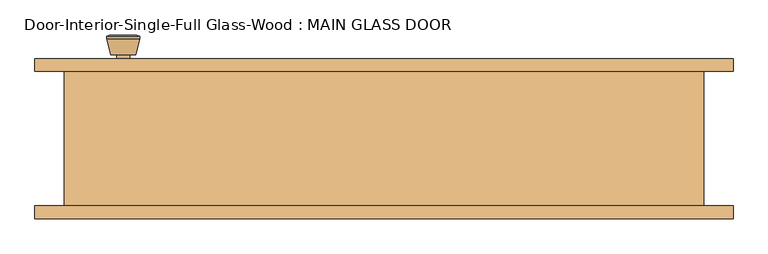
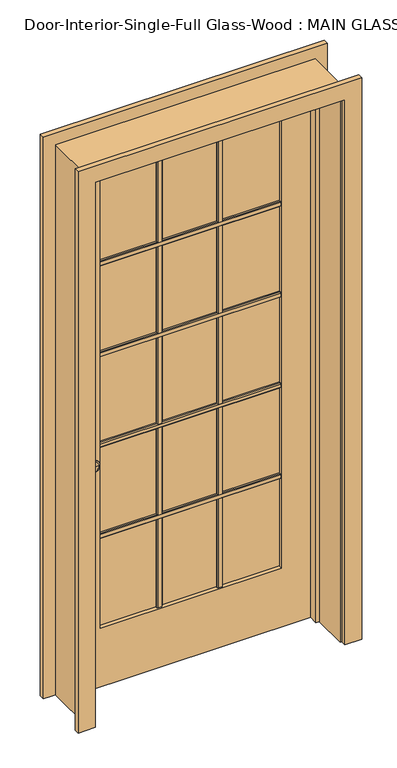
"""IFC4 building model written with IfcOpenShell, lengths in millimetres: door geometry, Door-Interior-Single-Full Glass-Wood : MAIN GLASS DOOR."""

from ifc_helpers import new_model, si_unit, point, frame, frame_2d, origin, place, context, project, spatial, polyline, circle_curve, trimmed, segment, composite_curve, outline, extrude, faceted_brep, source, transform, mapped, element, save
from ifc_brep_helpers import plane_surface, cylinder_surface, revolved_surface, advanced_brep


def door_interior_single_full_glass_wood_main_glass_door_aaee7461(model_context):
    return source(origin(), model_context, "Body", "SolidModel", [
        extrude(outline(polyline([(84.455, 1667.51), (90.805, 1667.51), (93.98, 1664.335), (93.98, 1651.635), (90.805, 1648.46), (84.455, 1648.46), (84.455, 1667.51)])), frame((-336.55, 0.0, 0.0), z_axis=(1.0, 0.0, 0.0), x_axis=(0.0, 1.0, 0.0)), (0.0, 0.0, 1.0), 673.1),
        extrude(outline(polyline([(84.455, 1310.9575), (90.805, 1310.9575), (93.98, 1307.7825), (93.98, 1295.0825), (90.805, 1291.9075), (84.455, 1291.9075), (84.455, 1310.9575)])), frame((-336.55, 0.0, 0.0), z_axis=(1.0, 0.0, 0.0), x_axis=(0.0, 1.0, 0.0)), (0.0, 0.0, 1.0), 673.1),
        extrude(outline(polyline([(84.455, 954.405), (90.805, 954.405), (93.98, 951.23), (93.98, 938.53), (90.805, 935.355), (84.455, 935.355), (84.455, 954.405)])), frame((-336.55, 0.0, 0.0), z_axis=(1.0, 0.0, 0.0), x_axis=(0.0, 1.0, 0.0)), (0.0, 0.0, 1.0), 673.1),
        extrude(outline(polyline([(84.455, 597.8525), (90.805, 597.8525), (93.98, 594.6775), (93.98, 581.9775), (90.805, 578.8025), (84.455, 578.8025), (84.455, 597.8525)])), frame((-336.55, 0.0, 0.0), z_axis=(1.0, 0.0, 0.0), x_axis=(0.0, 1.0, 0.0)), (0.0, 0.0, 1.0), 673.1),
        extrude(outline(polyline([(102.6583333, 84.455), (102.6583333, 90.805), (105.8333333, 93.98), (118.5333333, 93.98), (121.7083333, 90.805), (121.7083333, 84.455), (102.6583333, 84.455)])), frame((0.0, 0.0, 231.775), z_axis=(0.0, 0.0, 1.0), x_axis=(1.0, 0.0, 0.0)), (0.0, 0.0, 1.0), 1782.7625),
        extrude(outline(polyline([(-121.7083333, 84.455), (-121.7083333, 90.805), (-118.5333333, 93.98), (-105.8333333, 93.98), (-102.6583333, 90.805), (-102.6583333, 84.455), (-121.7083333, 84.455)])), frame((0.0, 0.0, 231.775), z_axis=(0.0, 0.0, 1.0), x_axis=(1.0, 0.0, 0.0)), (0.0, 0.0, 1.0), 1782.7625),
        extrude(outline(polyline([(77.47, 1667.51), (77.47, 1648.46), (71.12, 1648.46), (67.945, 1651.635), (67.945, 1664.335), (71.12, 1667.51), (77.47, 1667.51)])), frame((-336.55, 0.0, 0.0), z_axis=(1.0, 0.0, 0.0), x_axis=(0.0, 1.0, 0.0)), (0.0, 0.0, 1.0), 673.1),
        extrude(outline(polyline([(77.47, 1310.9575), (77.47, 1291.9075), (71.12, 1291.9075), (67.945, 1295.0825), (67.945, 1307.7825), (71.12, 1310.9575), (77.47, 1310.9575)])), frame((-336.55, 0.0, 0.0), z_axis=(1.0, 0.0, 0.0), x_axis=(0.0, 1.0, 0.0)), (0.0, 0.0, 1.0), 673.1),
        extrude(outline(polyline([(77.47, 954.405), (77.47, 935.355), (71.12, 935.355), (67.945, 938.53), (67.945, 951.23), (71.12, 954.405), (77.47, 954.405)])), frame((-336.55, 0.0, 0.0), z_axis=(1.0, 0.0, 0.0), x_axis=(0.0, 1.0, 0.0)), (0.0, 0.0, 1.0), 673.1),
        extrude(outline(polyline([(77.47, 597.8525), (77.47, 578.8025), (71.12, 578.8025), (67.945, 581.9775), (67.945, 594.6775), (71.12, 597.8525), (77.47, 597.8525)])), frame((-336.55, 0.0, 0.0), z_axis=(1.0, 0.0, 0.0), x_axis=(0.0, 1.0, 0.0)), (0.0, 0.0, 1.0), 673.1),
        extrude(outline(polyline([(102.6583333, 77.47), (121.7083333, 77.47), (121.7083333, 71.12), (118.5333333, 67.945), (105.8333333, 67.945), (102.6583333, 71.12), (102.6583333, 77.47)])), frame((0.0, 0.0, 231.775), z_axis=(0.0, 0.0, 1.0), x_axis=(1.0, 0.0, 0.0)), (0.0, 0.0, 1.0), 1782.7625),
        extrude(outline(polyline([(-121.7083333, 77.47), (-102.6583333, 77.47), (-102.6583333, 71.12), (-105.8333333, 67.945), (-118.5333333, 67.945), (-121.7083333, 71.12), (-121.7083333, 77.47)])), frame((0.0, 0.0, 231.775), z_axis=(0.0, 0.0, 1.0), x_axis=(1.0, 0.0, 0.0)), (0.0, 0.0, 1.0), 1782.7625),
        advanced_brep(
        [(-393.7, 57.5, 914.4), (-383.7, 57.5, 914.4), (-403.7, 57.5, 914.4), (-373.2241324, 8.5, 914.4), (-393.7, 8.5, 914.4), (-414.1758676, 8.5, 914.4), (-368.7, 10.3278681, 914.4), (-418.7, 10.3278681, 914.4), (-368.7, 13.7915463, 914.4), (-418.7, 13.7915463, 914.4), (-375.063764, 38.5, 914.4), (-412.336236, 38.5, 914.4), (-383.7, 38.5, 914.4), (-403.7, 38.5, 914.4)],
        [
            (0, 1),
            (1, 2, circle_curve(frame((-393.7, 57.5, 914.4), z_axis=(0.0, 1.0, 0.0), x_axis=(-1.0, 0.0, 0.0)), 10.0)),
            (2, 0),
            (2, 1, circle_curve(frame((-393.7, 57.5, 914.4), z_axis=(0.0, 1.0, 0.0), x_axis=(-1.0, 0.0, 0.0)), 10.0)),
            (3, 4),
            (4, 5),
            (5, 3, circle_curve(frame((-393.7, 8.5, 914.4), z_axis=(0.0, -1.0, 0.0), x_axis=(-1.0, 0.0, 0.0)), 20.4758676)),
            (3, 5, circle_curve(frame((-393.7, 8.5, 914.4), z_axis=(0.0, -1.0, 0.0), x_axis=(-1.0, 0.0, 0.0)), 20.4758676)),
            (6, 3),
            (5, 7),
            (7, 6, circle_curve(frame((-393.7, 10.3278681, 914.4), z_axis=(0.0, -1.0, 0.0), x_axis=(-1.0, 0.0, 0.0)), 25.0)),
            (6, 7, circle_curve(frame((-393.7, 10.3278681, 914.4), z_axis=(0.0, -1.0, 0.0), x_axis=(-1.0, 0.0, 0.0)), 25.0)),
            (8, 6),
            (7, 9),
            (9, 8, circle_curve(frame((-393.7, 13.7915463, 914.4), z_axis=(0.0, -1.0, 0.0), x_axis=(-1.0, 0.0, 0.0)), 25.0)),
            (8, 9, circle_curve(frame((-393.7, 13.7915463, 914.4), z_axis=(0.0, -1.0, 0.0), x_axis=(-1.0, 0.0, 0.0)), 25.0)),
            (10, 8),
            (9, 11),
            (11, 10, circle_curve(frame((-393.7, 38.5, 914.4), z_axis=(0.0, -1.0, 0.0), x_axis=(-1.0, 0.0, 0.0)), 18.636236)),
            (10, 11, circle_curve(frame((-393.7, 38.5, 914.4), z_axis=(0.0, -1.0, 0.0), x_axis=(-1.0, 0.0, 0.0)), 18.636236)),
            (12, 10),
            (11, 13),
            (13, 12, circle_curve(frame((-393.7, 38.5, 914.4), z_axis=(0.0, -1.0, 0.0), x_axis=(-1.0, 0.0, 0.0)), 10.0)),
            (12, 13, circle_curve(frame((-393.7, 38.5, 914.4), z_axis=(0.0, -1.0, 0.0), x_axis=(-1.0, 0.0, 0.0)), 10.0)),
            (1, 12),
            (13, 2),
        ],
        [
            plane_surface(frame((-393.7, 57.5, 914.4), z_axis=(0.0, 1.0, 0.0), x_axis=(-1.0, 0.0, 0.0))),
            plane_surface(frame((-393.7, 8.5, 914.4), z_axis=(0.0, -1.0, 0.0), x_axis=(-1.0, 0.0, 0.0))),
            revolved_surface(polyline([(-414.1758676, 8.5, 914.4), (-418.7, 10.3278681, 914.4)]), (-393.7, 57.5, 914.4), (0.0, 1.0, 0.0)),
            cylinder_surface(frame((-393.7, 57.5, 914.4), z_axis=(0.0, 1.0, 0.0), x_axis=(-1.0, 0.0, 0.0)), 25.0),
            revolved_surface(polyline([(-418.7, 13.7915463, 914.4), (-412.336236, 38.5, 914.4)]), (-393.7, 57.5, 914.4), (0.0, 1.0, 0.0)),
            plane_surface(frame((-393.7, 38.5, 914.4), z_axis=(0.0, 1.0, 0.0), x_axis=(-1.0, 0.0, 0.0))),
            cylinder_surface(frame((-393.7, 57.5, 914.4), z_axis=(0.0, 1.0, 0.0), x_axis=(-1.0, 0.0, 0.0)), 10.0),
        ],
        [
            (0, [[1, 2, 3]]),
            (0, [[-3, 4, -1]]),
            (1, [[5, 6, 7]]),
            (1, [[-6, -5, 8]]),
            (2, [[9, -7, 10, 11]]),
            (2, [[-10, -8, -9, 12]]),
            (3, [[13, -11, 14, 15]]),
            (3, [[-14, -12, -13, 16]]),
            (4, [[17, -15, 18, 19]]),
            (4, [[-18, -16, -17, 20]]),
            (5, [[21, -19, 22, 23]]),
            (5, [[-22, -20, -21, 24]]),
            (6, [[25, -23, 26, -2]]),
            (6, [[-26, -24, -25, -4]]),
        ],
    ),
        extrude(outline(composite_curve([segment(trimmed(circle_curve(frame_2d((914.4, -393.7)), 30.0), [point((914.4, -423.7))], [point((914.4, -363.7))], False, "CARTESIAN"), True, "CONTINUOUS"), segment(trimmed(circle_curve(frame_2d((914.4, -393.7)), 30.0), [point((914.4, -363.7))], [point((914.4, -423.7))], False, "CARTESIAN"), True, "CONTINUOUS")], self_intersect=False)), frame((0.0, 57.5, 0.0), z_axis=(0.0, 1.0, 0.0), x_axis=(0.0, 0.0, 1.0)), (0.0, 0.0, 1.0), 6.0),
        advanced_brep(
        [(-393.7, 104.425, 914.4), (-403.7, 104.425, 914.4), (-383.7, 104.425, 914.4), (-373.2241324, 153.425, 914.4), (-414.1758676, 153.425, 914.4), (-393.7, 153.425, 914.4), (-368.7, 151.5971319, 914.4), (-418.7, 151.5971319, 914.4), (-368.7, 148.1334537, 914.4), (-418.7, 148.1334537, 914.4), (-375.063764, 123.425, 914.4), (-412.336236, 123.425, 914.4), (-383.7, 123.425, 914.4), (-403.7, 123.425, 914.4)],
        [
            (0, 1),
            (1, 2, circle_curve(frame((-393.7, 104.425, 914.4), z_axis=(0.0, -1.0, 0.0), x_axis=(-1.0, 0.0, 0.0)), 10.0)),
            (2, 0),
            (2, 1, circle_curve(frame((-393.7, 104.425, 914.4), z_axis=(0.0, -1.0, 0.0), x_axis=(-1.0, 0.0, 0.0)), 10.0)),
            (3, 4, circle_curve(frame((-393.7, 153.425, 914.4), z_axis=(0.0, 1.0, 0.0), x_axis=(-1.0, 0.0, 0.0)), 20.4758676)),
            (4, 5),
            (5, 3),
            (4, 3, circle_curve(frame((-393.7, 153.425, 914.4), z_axis=(0.0, 1.0, 0.0), x_axis=(-1.0, 0.0, 0.0)), 20.4758676)),
            (6, 7, circle_curve(frame((-393.7, 151.5971319, 914.4), z_axis=(0.0, 1.0, 0.0), x_axis=(-1.0, 0.0, 0.0)), 25.0)),
            (7, 4),
            (3, 6),
            (7, 6, circle_curve(frame((-393.7, 151.5971319, 914.4), z_axis=(0.0, 1.0, 0.0), x_axis=(-1.0, 0.0, 0.0)), 25.0)),
            (8, 9, circle_curve(frame((-393.7, 148.1334537, 914.4), z_axis=(0.0, 1.0, 0.0), x_axis=(-1.0, 0.0, 0.0)), 25.0)),
            (9, 7),
            (6, 8),
            (9, 8, circle_curve(frame((-393.7, 148.1334537, 914.4), z_axis=(0.0, 1.0, 0.0), x_axis=(-1.0, 0.0, 0.0)), 25.0)),
            (10, 11, circle_curve(frame((-393.7, 123.425, 914.4), z_axis=(0.0, 1.0, 0.0), x_axis=(-1.0, 0.0, 0.0)), 18.636236)),
            (11, 9),
            (8, 10),
            (11, 10, circle_curve(frame((-393.7, 123.425, 914.4), z_axis=(0.0, 1.0, 0.0), x_axis=(-1.0, 0.0, 0.0)), 18.636236)),
            (12, 13, circle_curve(frame((-393.7, 123.425, 914.4), z_axis=(0.0, 1.0, 0.0), x_axis=(-1.0, 0.0, 0.0)), 10.0)),
            (13, 11),
            (10, 12),
            (13, 12, circle_curve(frame((-393.7, 123.425, 914.4), z_axis=(0.0, 1.0, 0.0), x_axis=(-1.0, 0.0, 0.0)), 10.0)),
            (1, 13),
            (12, 2),
        ],
        [
            plane_surface(frame((-393.7, 104.425, 914.4), z_axis=(0.0, -1.0, 0.0), x_axis=(-1.0, 0.0, 0.0))),
            plane_surface(frame((-393.7, 153.425, 914.4), z_axis=(0.0, 1.0, 0.0), x_axis=(-1.0, 0.0, 0.0))),
            revolved_surface(polyline([(-414.1758676, 153.425, 914.4), (-418.7, 151.5971319, 914.4)]), (-393.7, 104.425, 914.4), (0.0, -1.0, 0.0)),
            cylinder_surface(frame((-393.7, 104.425, 914.4), z_axis=(0.0, -1.0, 0.0), x_axis=(-1.0, 0.0, 0.0)), 25.0),
            revolved_surface(polyline([(-418.7, 148.1334537, 914.4), (-412.336236, 123.425, 914.4)]), (-393.7, 104.425, 914.4), (0.0, -1.0, 0.0)),
            plane_surface(frame((-393.7, 123.425, 914.4), z_axis=(0.0, -1.0, 0.0), x_axis=(-1.0, 0.0, 0.0))),
            cylinder_surface(frame((-393.7, 104.425, 914.4), z_axis=(0.0, -1.0, 0.0), x_axis=(-1.0, 0.0, 0.0)), 10.0),
        ],
        [
            (0, [[1, 2, 3]]),
            (0, [[-3, 4, -1]]),
            (1, [[5, 6, 7]]),
            (1, [[8, -7, -6]]),
            (2, [[9, 10, -5, 11]]),
            (2, [[12, -11, -8, -10]]),
            (3, [[13, 14, -9, 15]]),
            (3, [[16, -15, -12, -14]]),
            (4, [[17, 18, -13, 19]]),
            (4, [[20, -19, -16, -18]]),
            (5, [[21, 22, -17, 23]]),
            (5, [[24, -23, -20, -22]]),
            (6, [[-2, 25, -21, 26]]),
            (6, [[-4, -26, -24, -25]]),
        ],
    ),
        extrude(outline(composite_curve([segment(trimmed(circle_curve(frame_2d((914.4, -393.7)), 30.0), [point((914.4, -423.7))], [point((914.4, -363.7))], False, "CARTESIAN"), True, "CONTINUOUS"), segment(trimmed(circle_curve(frame_2d((914.4, -393.7)), 30.0), [point((914.4, -363.7))], [point((914.4, -423.7))], False, "CARTESIAN"), True, "CONTINUOUS")], self_intersect=False)), frame((0.0, 98.425, 0.0), z_axis=(0.0, 1.0, 0.0), x_axis=(0.0, 0.0, 1.0)), (0.0, 0.0, 1.0), 6.0),
        faceted_brep([(482.6, 98.425, 0.0), (482.6, -104.775, 0.0), (457.2, -104.775, 0.0), (457.2, 28.575, 0.0), (444.5, 28.575, 0.0), (444.5, 63.5, 0.0), (457.2, 63.5, 0.0), (457.2, 98.425, 0.0), (482.6, 98.425, 2159.0), (482.6, -104.775, 2159.0), (-482.6, -104.775, 2159.0), (-482.6, -104.775, 0.0), (-457.2, -104.775, 0.0), (-457.2, -104.775, 2133.6), (457.2, -104.775, 2133.6), (457.2, 28.575, 2133.6), (-457.2, 28.575, 2133.6), (-457.2, 28.575, 0.0), (-444.5, 28.575, 0.0), (-444.5, 28.575, 2120.9), (444.5, 28.575, 2120.9), (444.5, 63.5, 2120.9), (-444.5, 63.5, 2120.9), (-444.5, 63.5, 0.0), (-457.2, 63.5, 0.0), (-457.2, 63.5, 2133.6), (457.2, 63.5, 2133.6), (457.2, 98.425, 2133.6), (-457.2, 98.425, 2133.6), (-457.2, 98.425, 0.0), (-482.6, 98.425, 0.0), (-482.6, 98.425, 2159.0)], [[[0, 1, 2, 3, 4, 5, 6, 7]], [[1, 0, 8, 9]], [[2, 1, 9, 10, 11, 12, 13, 14]], [[3, 2, 14, 15]], [[4, 3, 15, 16, 17, 18, 19, 20]], [[5, 4, 20, 21]], [[6, 5, 21, 22, 23, 24, 25, 26]], [[7, 6, 26, 27]], [[0, 7, 27, 28, 29, 30, 31, 8]], [[9, 8, 31, 10]], [[15, 14, 13, 16]], [[21, 20, 19, 22]], [[27, 26, 25, 28]], [[30, 29, 24, 23, 18, 17, 12, 11]], [[10, 31, 30, 11]], [[16, 13, 12, 17]], [[22, 19, 18, 23]], [[28, 25, 24, 29]]]),
        extrude(outline(polyline([(2133.6, -457.2), (0.0, -457.2), (0.0, 457.2), (2133.6, 457.2), (2133.6, -457.2)]), holes=[polyline([(2014.5375, -336.55), (2014.5375, 336.55), (231.775, 336.55), (231.775, -336.55), (2014.5375, -336.55)])]), frame((0.0, 63.5, 0.0), z_axis=(0.0, 1.0, 0.0), x_axis=(0.0, 0.0, 1.0)), (0.0, 0.0, 1.0), 34.925),
        extrude(outline(polyline([(336.55, 77.47), (-336.55, 77.47), (-336.55, 84.455), (336.55, 84.455), (336.55, 77.47)])), frame((0.0, 0.0, 231.775), z_axis=(0.0, 0.0, 1.0), x_axis=(1.0, 0.0, 0.0)), (0.0, 0.0, 1.0), 1782.7625),
        extrude(outline(polyline([(0.0, 463.55), (0.0, 527.05), (2203.45, 527.05), (2203.45, -527.05), (0.0, -527.05), (0.0, -463.55), (2139.95, -463.55), (2139.95, 463.55), (0.0, 463.55)])), frame((0.0, 98.425, 0.0), z_axis=(0.0, 1.0, 0.0), x_axis=(0.0, 0.0, 1.0)), (0.0, 0.0, 1.0), 19.05),
        extrude(outline(polyline([(0.0, 463.55), (0.0, 527.05), (2203.45, 527.05), (2203.45, -527.05), (0.0, -527.05), (0.0, -463.55), (2139.95, -463.55), (2139.95, 463.55), (0.0, 463.55)])), frame((0.0, -123.825, 0.0), z_axis=(0.0, 1.0, 0.0), x_axis=(0.0, 0.0, 1.0)), (0.0, 0.0, 1.0), 19.05),
    ])


if __name__ == "__main__":
    model = new_model("IFC4")
    model_context = context("Model", 3, world=origin())
    ifc_project = project(units=[si_unit("LENGTHUNIT", "METRE", prefix="MILLI")], contexts=[model_context])
    site = spatial("IfcSite", under=ifc_project)
    building = spatial("IfcBuilding", under=site)
    placement = place(None, origin())
    door_interior_single_full_glass_wood_main_glass_door_shape = door_interior_single_full_glass_wood_main_glass_door_aaee7461(model_context)
    element("IfcDoor", 1, ObjectType="Door-Interior-Single-Full Glass-Wood : MAIN GLASS DOOR", at=placement, inside=building, context=model_context, shape_type="MappedRepresentation", body=[
        mapped(door_interior_single_full_glass_wood_main_glass_door_shape, transform((0.0, 0.0, 0.0), x_axis=(1.0, 0.0, 0.0), y_axis=(0.0, 1.0, 0.0), z_axis=(0.0, 0.0, 1.0))),
    ])
    save(model, "model.ifc")

# Revit data of these elements
# Type "Door-Interior-Single-Full Glass-Wood : MAIN GLASS DOOR"
#   Type Mark = "9"
#   Assembly Code = "C1020300"
#   Analytic Construction = "Wood frame with single clear glass"
#   Top Rail = 0' - 4 11/16"
#   Thickness = 0' - 1 3/8"
#   Thermal Resistance (R) = 1.0102 (h·ft²·°F)/BTU
#   Swing Angle [instance default] = 90.00°
#   Stiles = 0' - 4 3/4"
#   Rough Width = 3' - 2"
#   Rough Height = 7' - 1"
#   Height = 7' - 0"
#   Width = 3' - 0"
#   Heat Transfer Coefficient (U) = 0.9900 BTU/(h·ft²·°F)
#   Bottom Rail = 0' - 9 1/8"
#   Show Grill [instance default] = yes
#   Trim Material = Cherry
#   Panel Material = Cherry
#   Frame Material = Cherry
#   Door Handle Material = Aluminum
#   Visual Light Transmittance = 0
#   Solar Heat Gain Coefficient = 0
#   Wall Closure = (empty or 0)
#   Function = (empty or 0)
# Element 1 (IfcDoor, "Door-Interior-Single-Full Glass-Wood : MAIN GLASS DOOR")
#   Materials on its faces: "Cherry", "Aluminum", "Glass"
# Materials
#   "Cherry": class "Wood", colour RGB 226 177 128, transparency 0, Description = "Prunus Serotina", Cost = 0
#   "Aluminum": class "Metal", colour RGB 247 247 247, transparency 0, Description = "Aluminum 6061", Cost = 0
#   "Glass": class "Glass", colour RGB 0 128 192, transparency 0.75, Description = "Soda Lime Glass", Cost = 0
